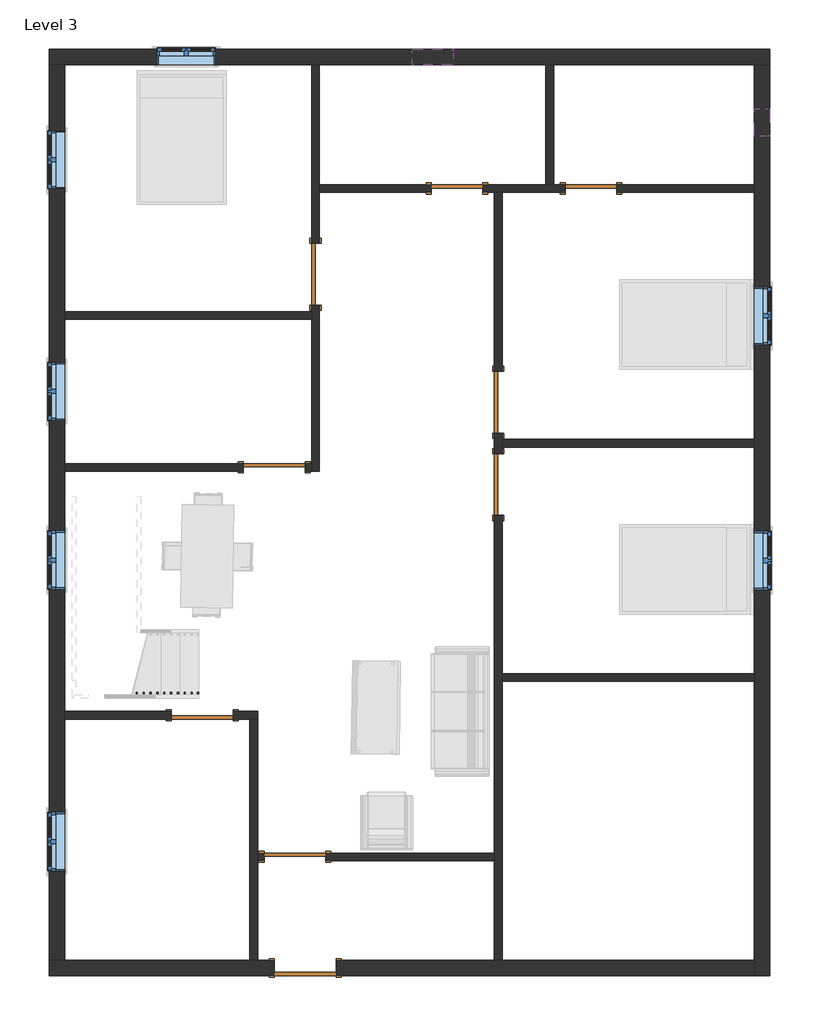
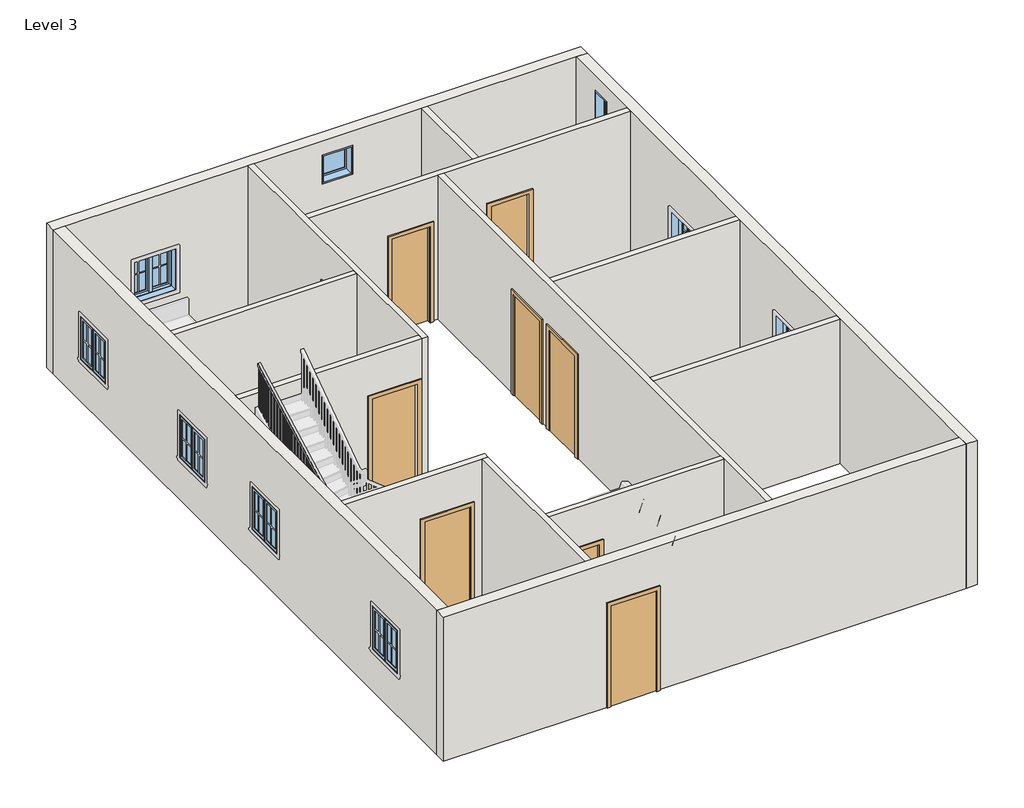
# One storey, part 1 of 2: 15 walls, 9 doors, 9 windows, 1 railing.
"""IFC4 building model written with IfcOpenShell, lengths in millimetres."""

from ifc_helpers import new_model, si_unit, frame, origin, place, context, project, spatial, polyline, outline, extrude, faceted_brep, transform, mapped, element, save
from components import door_d8f5dbb5, door_f2b275c1, door_305aa2a5, door_e5f9f3c4, door_0ca8825f, window_aa618e30, window_80340324, window_339605e1

model = new_model("IFC4")

# Units and contexts
model_context = context("Model", 3, world=origin())
ifc_project = project(units=[si_unit("LENGTHUNIT", "METRE", prefix="MILLI")], contexts=[model_context])

# Site, building, storey
site = spatial("IfcSite", under=ifc_project)
building = spatial("IfcBuilding", under=site)
storey = spatial("IfcBuildingStorey", under=building, Name="Level 3", Elevation=3200.4)

# Doors
placement = place(None, origin())
door_shape = door_d8f5dbb5(model_context)
element("IfcDoor", 1, ObjectType="Single-Flush : 30\" x 80\"", at=placement, inside=storey, context=model_context, shape_type="MappedRepresentation", body=[
    mapped(door_shape, transform((-551.6099931, 5332.4435985, 3200.4), x_axis=(1.0, 0.0, 0.0), y_axis=(0.0, 1.0, 0.0), z_axis=(0.0, 0.0, 1.0))),
])
door_2_shape = door_f2b275c1(model_context)
element("IfcDoor", 2, ObjectType="Single-Flush : 30\" x 80\"", at=placement, inside=storey, context=model_context, shape_type="MappedRepresentation", body=[
    mapped(door_2_shape, transform((1429.5900069, 5332.4435985, 3200.4), x_axis=(-1.0, 0.0, 0.0), y_axis=(0.0, -1.0, 0.0), z_axis=(0.0, 0.0, 1.0))),
])
door_3_shape = door_305aa2a5(model_context)
element("IfcDoor", 3, ObjectType="Single-Flush : 36\" x 84\"", at=placement, inside=storey, context=model_context, shape_type="MappedRepresentation", body=[
    mapped(door_3_shape, transform((-2647.1099931, 4062.4435985, 3200.4), x_axis=(0.0, -1.0, 0.0), y_axis=(1.0, 0.0, 0.0), z_axis=(0.0, 0.0, 1.0))),
])
element("IfcDoor", 4, ObjectType="Single-Flush : 36\" x 84\"", at=placement, inside=storey, context=model_context, shape_type="MappedRepresentation", body=[
    mapped(door_3_shape, transform((57.9900069, 2170.1435985, 3200.4), x_axis=(0.0, -1.0, 0.0), y_axis=(1.0, 0.0, 0.0), z_axis=(0.0, 0.0, 1.0))),
])
element("IfcDoor", 5, ObjectType="Single-Flush : 36\" x 84\"", at=placement, inside=storey, context=model_context, shape_type="MappedRepresentation", body=[
    mapped(door_3_shape, transform((-4323.5099931, -2465.3564015, 3200.4), x_axis=(1.0, 0.0, 0.0), y_axis=(0.0, 1.0, 0.0), z_axis=(0.0, 0.0, 1.0))),
])
element("IfcDoor", 6, ObjectType="Single-Flush : 36\" x 84\"", at=placement, inside=storey, context=model_context, shape_type="MappedRepresentation", body=[
    mapped(door_3_shape, transform((-2951.9099931, -4560.8564015, 3200.4), x_axis=(-1.0, 0.0, 0.0), y_axis=(0.0, -1.0, 0.0), z_axis=(0.0, 0.0, 1.0))),
])
door_4_shape = door_e5f9f3c4(model_context)
element("IfcDoor", 7, ObjectType="Single-Flush : 36\" x 84\"", at=placement, inside=storey, context=model_context, shape_type="MappedRepresentation", body=[
    mapped(door_4_shape, transform((-3256.7099931, 1204.9435985, 3200.4), x_axis=(1.0, 0.0, 0.0), y_axis=(0.0, 1.0, 0.0), z_axis=(0.0, 0.0, 1.0))),
])
element("IfcDoor", 8, ObjectType="Single-Flush : 36\" x 84\"", at=placement, inside=storey, context=model_context, shape_type="MappedRepresentation", body=[
    mapped(door_4_shape, transform((57.9900069, 950.9435985, 3200.4), x_axis=(0.0, 1.0, 0.0), y_axis=(-1.0, 0.0, 0.0), z_axis=(0.0, 0.0, 1.0))),
])
door_5_shape = door_0ca8825f(model_context)
element("IfcDoor", 9, ObjectType="Single-Flush : 36\" x 84\"", at=placement, inside=storey, context=model_context, shape_type="MappedRepresentation", body=[
    mapped(door_5_shape, transform((-2799.5099931, -6205.5064015, 3200.4), x_axis=(-1.0, 0.0, 0.0), y_axis=(0.0, -1.0, 0.0), z_axis=(0.0, 0.0, 1.0))),
])

# Railing
element("IfcRailing", 10, ObjectType="Handrail - Rectangular", at=placement, inside=storey, context=model_context, shape_type="SolidModel", body=[
    faceted_brep([(-4378.4230036, -2160.5564015, 4961.4666667), (-4378.4230036, -2160.5564015, 4905.3107192), (-4378.4230036, -2109.7564015, 4905.3107192), (-4378.4230036, -2109.7564015, 4961.4666667), (-5973.5005957, -2160.5564015, 5712.9835228), (-5984.8684735, -2160.5564015, 5662.1835228), (-5984.8684735, -2109.7564015, 5662.1835228), (-5973.5005957, -2109.7564015, 5712.9835228), (-6196.7599931, -2160.5564015, 5712.9835228), (-6196.7599931, -2160.5564015, 5662.1835228), (-6145.9599931, -2109.7564015, 5662.1835228), (-6145.9599931, -2109.7564015, 5712.9835228), (-6196.7599931, -1959.3194067, 5712.9835228), (-6196.7599931, -1946.6862419, 5662.1835228), (-6145.9599931, -1946.6862419, 5662.1835228), (-6145.9599931, -1959.3194067, 5712.9835228), (-6196.7599931, 775.380588, 7162.8), (-6145.9599931, 775.380588, 7162.8), (-6145.9599931, 775.380588, 7105.3024571), (-6196.7599931, 775.380588, 7105.3024571)], [[[0, 1, 2, 3]], [[1, 0, 4, 5]], [[2, 1, 5, 6]], [[3, 2, 6, 7]], [[0, 3, 7, 4]], [[5, 4, 8, 9]], [[6, 5, 9, 10]], [[7, 6, 10, 11]], [[4, 7, 11, 8]], [[9, 8, 12, 13]], [[10, 9, 13, 14]], [[11, 10, 14, 15]], [[8, 11, 15, 12]], [[16, 17, 18, 19]], [[13, 12, 16, 19]], [[14, 13, 19, 18]], [[15, 14, 18, 17]], [[12, 15, 17, 16]]]),
    extrude(outline(polyline([(719.1685985, 7075.5013569), (719.1685985, 6079.0666667), (700.1185985, 6079.0666667), (700.1185985, 7065.401893), (719.1685985, 7075.5013569)])), frame((-6180.8849931, 0.0, 0.0), z_axis=(1.0, 0.0, 0.0), x_axis=(0.0, 1.0, 0.0)), (0.0, 0.0, 1.0), 19.05),
    extrude(outline(polyline([(617.5685985, 7021.6375494), (617.5685985, 6079.0666667), (598.5185985, 6079.0666667), (598.5185985, 7011.5380855), (617.5685985, 7021.6375494)])), frame((-6180.8849931, 0.0, 0.0), z_axis=(1.0, 0.0, 0.0), x_axis=(0.0, 1.0, 0.0)), (0.0, 0.0, 1.0), 19.05),
    extrude(outline(polyline([(515.9685985, 6967.7737419), (515.9685985, 6079.0666667), (496.9185985, 6079.0666667), (496.9185985, 6957.674278), (515.9685985, 6967.7737419)])), frame((-6180.8849931, 0.0, 0.0), z_axis=(1.0, 0.0, 0.0), x_axis=(0.0, 1.0, 0.0)), (0.0, 0.0, 1.0), 19.05),
    extrude(outline(polyline([(414.3685985, 6913.9099344), (414.3685985, 5909.7333333), (395.3185985, 5909.7333333), (395.3185985, 6903.8104705), (414.3685985, 6913.9099344)])), frame((-6180.8849931, 0.0, 0.0), z_axis=(1.0, 0.0, 0.0), x_axis=(0.0, 1.0, 0.0)), (0.0, 0.0, 1.0), 19.05),
    extrude(outline(polyline([(312.7685985, 6860.0461269), (312.7685985, 5909.7333333), (293.7185985, 5909.7333333), (293.7185985, 6849.946663), (312.7685985, 6860.0461269)])), frame((-6180.8849931, 0.0, 0.0), z_axis=(1.0, 0.0, 0.0), x_axis=(0.0, 1.0, 0.0)), (0.0, 0.0, 1.0), 19.05),
    extrude(outline(polyline([(211.1685985, 6806.1823194), (211.1685985, 5740.4), (192.1185985, 5740.4), (192.1185985, 6796.0828555), (211.1685985, 6806.1823194)])), frame((-6180.8849931, 0.0, 0.0), z_axis=(1.0, 0.0, 0.0), x_axis=(0.0, 1.0, 0.0)), (0.0, 0.0, 1.0), 19.05),
    extrude(outline(polyline([(109.5685985, 6752.3185119), (109.5685985, 5740.4), (90.5185985, 5740.4), (90.5185985, 6742.219048), (109.5685985, 6752.3185119)])), frame((-6180.8849931, 0.0, 0.0), z_axis=(1.0, 0.0, 0.0), x_axis=(0.0, 1.0, 0.0)), (0.0, 0.0, 1.0), 19.05),
    extrude(outline(polyline([(7.9685985, 6698.4547044), (7.9685985, 5740.4), (-11.0814015, 5740.4), (-11.0814015, 6688.3552405), (7.9685985, 6698.4547044)])), frame((-6180.8849931, 0.0, 0.0), z_axis=(1.0, 0.0, 0.0), x_axis=(0.0, 1.0, 0.0)), (0.0, 0.0, 1.0), 19.05),
    extrude(outline(polyline([(-93.6314015, 6644.5908969), (-93.6314015, 5571.0666667), (-112.6814015, 5571.0666667), (-112.6814015, 6634.491433), (-93.6314015, 6644.5908969)])), frame((-6180.8849931, 0.0, 0.0), z_axis=(1.0, 0.0, 0.0), x_axis=(0.0, 1.0, 0.0)), (0.0, 0.0, 1.0), 19.05),
    extrude(outline(polyline([(-195.2314015, 6590.7270894), (-195.2314015, 5571.0666667), (-214.2814015, 5571.0666667), (-214.2814015, 6580.6276255), (-195.2314015, 6590.7270894)])), frame((-6180.8849931, 0.0, 0.0), z_axis=(1.0, 0.0, 0.0), x_axis=(0.0, 1.0, 0.0)), (0.0, 0.0, 1.0), 19.05),
    extrude(outline(polyline([(-296.8314015, 6536.8632819), (-296.8314015, 5571.0666667), (-315.8814015, 5571.0666667), (-315.8814015, 6526.763818), (-296.8314015, 6536.8632819)])), frame((-6180.8849931, 0.0, 0.0), z_axis=(1.0, 0.0, 0.0), x_axis=(0.0, 1.0, 0.0)), (0.0, 0.0, 1.0), 19.05),
    extrude(outline(polyline([(-398.4314015, 6482.9994744), (-398.4314015, 5401.7333333), (-417.4814015, 5401.7333333), (-417.4814015, 6472.9000105), (-398.4314015, 6482.9994744)])), frame((-6180.8849931, 0.0, 0.0), z_axis=(1.0, 0.0, 0.0), x_axis=(0.0, 1.0, 0.0)), (0.0, 0.0, 1.0), 19.05),
    extrude(outline(polyline([(-500.0314015, 6429.1356669), (-500.0314015, 5401.7333333), (-519.0814015, 5401.7333333), (-519.0814015, 6419.036203), (-500.0314015, 6429.1356669)])), frame((-6180.8849931, 0.0, 0.0), z_axis=(1.0, 0.0, 0.0), x_axis=(0.0, 1.0, 0.0)), (0.0, 0.0, 1.0), 19.05),
    extrude(outline(polyline([(-601.6314015, 6375.2718594), (-601.6314015, 5401.7333333), (-620.6814015, 5401.7333333), (-620.6814015, 6365.1723955), (-601.6314015, 6375.2718594)])), frame((-6180.8849931, 0.0, 0.0), z_axis=(1.0, 0.0, 0.0), x_axis=(0.0, 1.0, 0.0)), (0.0, 0.0, 1.0), 19.05),
    extrude(outline(polyline([(-703.2314015, 6321.4080519), (-703.2314015, 5232.4), (-722.2814015, 5232.4), (-722.2814015, 6311.308588), (-703.2314015, 6321.4080519)])), frame((-6180.8849931, 0.0, 0.0), z_axis=(1.0, 0.0, 0.0), x_axis=(0.0, 1.0, 0.0)), (0.0, 0.0, 1.0), 19.05),
    extrude(outline(polyline([(-804.8314015, 6267.5442444), (-804.8314015, 5232.4), (-823.8814015, 5232.4), (-823.8814015, 6257.4447805), (-804.8314015, 6267.5442444)])), frame((-6180.8849931, 0.0, 0.0), z_axis=(1.0, 0.0, 0.0), x_axis=(0.0, 1.0, 0.0)), (0.0, 0.0, 1.0), 19.05),
    extrude(outline(polyline([(-906.4314015, 6213.6804369), (-906.4314015, 5232.4), (-925.4814015, 5232.4), (-925.4814015, 6203.580973), (-906.4314015, 6213.6804369)])), frame((-6180.8849931, 0.0, 0.0), z_axis=(1.0, 0.0, 0.0), x_axis=(0.0, 1.0, 0.0)), (0.0, 0.0, 1.0), 19.05),
    extrude(outline(polyline([(-1008.0314015, 6159.8166294), (-1008.0314015, 5063.0666667), (-1027.0814015, 5063.0666667), (-1027.0814015, 6149.7171655), (-1008.0314015, 6159.8166294)])), frame((-6180.8849931, 0.0, 0.0), z_axis=(1.0, 0.0, 0.0), x_axis=(0.0, 1.0, 0.0)), (0.0, 0.0, 1.0), 19.05),
    extrude(outline(polyline([(-1109.6314015, 6105.9528219), (-1109.6314015, 5063.0666667), (-1128.6814015, 5063.0666667), (-1128.6814015, 6095.853358), (-1109.6314015, 6105.9528219)])), frame((-6180.8849931, 0.0, 0.0), z_axis=(1.0, 0.0, 0.0), x_axis=(0.0, 1.0, 0.0)), (0.0, 0.0, 1.0), 19.05),
    extrude(outline(polyline([(-1211.2314015, 6052.0890144), (-1211.2314015, 5063.0666667), (-1230.2814015, 5063.0666667), (-1230.2814015, 6041.9895505), (-1211.2314015, 6052.0890144)])), frame((-6180.8849931, 0.0, 0.0), z_axis=(1.0, 0.0, 0.0), x_axis=(0.0, 1.0, 0.0)), (0.0, 0.0, 1.0), 19.05),
    extrude(outline(polyline([(-1312.8314015, 5998.2252069), (-1312.8314015, 5063.0666667), (-1331.8814015, 5063.0666667), (-1331.8814015, 5988.125743), (-1312.8314015, 5998.2252069)])), frame((-6180.8849931, 0.0, 0.0), z_axis=(1.0, 0.0, 0.0), x_axis=(0.0, 1.0, 0.0)), (0.0, 0.0, 1.0), 19.05),
    extrude(outline(polyline([(-1414.4314015, 5944.3613994), (-1414.4314015, 4893.7333333), (-1433.4814015, 4893.7333333), (-1433.4814015, 5934.2619355), (-1414.4314015, 5944.3613994)])), frame((-6180.8849931, 0.0, 0.0), z_axis=(1.0, 0.0, 0.0), x_axis=(0.0, 1.0, 0.0)), (0.0, 0.0, 1.0), 19.05),
    extrude(outline(polyline([(-1516.0314015, 5890.4975919), (-1516.0314015, 4893.7333333), (-1535.0814015, 4893.7333333), (-1535.0814015, 5880.398128), (-1516.0314015, 5890.4975919)])), frame((-6180.8849931, 0.0, 0.0), z_axis=(1.0, 0.0, 0.0), x_axis=(0.0, 1.0, 0.0)), (0.0, 0.0, 1.0), 19.05),
    extrude(outline(polyline([(-1617.6314015, 5836.6337844), (-1617.6314015, 4893.7333333), (-1636.6814015, 4893.7333333), (-1636.6814015, 5826.5343205), (-1617.6314015, 5836.6337844)])), frame((-6180.8849931, 0.0, 0.0), z_axis=(1.0, 0.0, 0.0), x_axis=(0.0, 1.0, 0.0)), (0.0, 0.0, 1.0), 19.05),
    extrude(outline(polyline([(-1719.2314015, 5782.7699769), (-1719.2314015, 4893.7333333), (-1738.2814015, 4893.7333333), (-1738.2814015, 5772.670513), (-1719.2314015, 5782.7699769)])), frame((-6180.8849931, 0.0, 0.0), z_axis=(1.0, 0.0, 0.0), x_axis=(0.0, 1.0, 0.0)), (0.0, 0.0, 1.0), 19.05),
    extrude(outline(polyline([(-1820.8314015, 5728.9061694), (-1820.8314015, 4724.4), (-1839.8814015, 4724.4), (-1839.8814015, 5718.8067055), (-1820.8314015, 5728.9061694)])), frame((-6180.8849931, 0.0, 0.0), z_axis=(1.0, 0.0, 0.0), x_axis=(0.0, 1.0, 0.0)), (0.0, 0.0, 1.0), 19.05),
    extrude(outline(polyline([(-1922.4314015, 5675.0423619), (-1922.4314015, 4724.4), (-1941.4814015, 4724.4), (-1941.4814015, 5664.942898), (-1922.4314015, 5675.0423619)])), frame((-6180.8849931, 0.0, 0.0), z_axis=(1.0, 0.0, 0.0), x_axis=(0.0, 1.0, 0.0)), (0.0, 0.0, 1.0), 19.05),
    extrude(outline(polyline([(-6180.8849931, -2043.0814015), (-6180.8849931, -2024.0314015), (-6161.8349931, -2024.0314015), (-6161.8349931, -2043.0814015), (-6180.8849931, -2043.0814015)])), frame((0.0, 0.0, 4724.4), z_axis=(0.0, 0.0, 1.0), x_axis=(1.0, 0.0, 0.0)), (0.0, 0.0, 1.0), 937.7835228),
    extrude(outline(polyline([(-6096.0980036, -2144.6814015), (-6115.1480036, -2144.6814015), (-6115.1480036, -2125.6314015), (-6096.0980036, -2125.6314015), (-6096.0980036, -2144.6814015)])), frame((0.0, 0.0, 4724.4), z_axis=(0.0, 0.0, 1.0), x_axis=(1.0, 0.0, 0.0)), (0.0, 0.0, 1.0), 937.7835228),
    extrude(outline(polyline([(-5994.4980036, -2144.6814015), (-6013.5480036, -2144.6814015), (-6013.5480036, -2125.6314015), (-5994.4980036, -2125.6314015), (-5994.4980036, -2144.6814015)])), frame((0.0, 0.0, 4724.4), z_axis=(0.0, 0.0, 1.0), x_axis=(1.0, 0.0, 0.0)), (0.0, 0.0, 1.0), 937.7835228),
    extrude(outline(polyline([(5627.827224, -5911.9480036), (4724.4, -5911.9480036), (4724.4, -5892.8980036), (5618.8518637, -5892.8980036), (5627.827224, -5911.9480036)])), frame((0.0, -2144.6814015, 0.0), z_axis=(0.0, 1.0, 0.0), x_axis=(0.0, 0.0, 1.0)), (0.0, 0.0, 1.0), 19.05),
    extrude(outline(polyline([(5579.9586357, -5810.3480036), (4724.4, -5810.3480036), (4724.4, -5791.2980036), (5570.9832754, -5791.2980036), (5579.9586357, -5810.3480036)])), frame((0.0, -2144.6814015, 0.0), z_axis=(0.0, 1.0, 0.0), x_axis=(0.0, 0.0, 1.0)), (0.0, 0.0, 1.0), 19.05),
    extrude(outline(polyline([(5532.0900474, -5708.7480036), (4555.0666667, -5708.7480036), (4555.0666667, -5689.6980036), (5523.1146871, -5689.6980036), (5532.0900474, -5708.7480036)])), frame((0.0, -2144.6814015, 0.0), z_axis=(0.0, 1.0, 0.0), x_axis=(0.0, 0.0, 1.0)), (0.0, 0.0, 1.0), 19.05),
    extrude(outline(polyline([(5484.2214591, -5607.1480036), (4555.0666667, -5607.1480036), (4555.0666667, -5588.0980036), (5475.2460988, -5588.0980036), (5484.2214591, -5607.1480036)])), frame((0.0, -2144.6814015, 0.0), z_axis=(0.0, 1.0, 0.0), x_axis=(0.0, 0.0, 1.0)), (0.0, 0.0, 1.0), 19.05),
    extrude(outline(polyline([(5436.3528708, -5505.5480036), (4555.0666667, -5505.5480036), (4555.0666667, -5486.4980036), (5427.3775105, -5486.4980036), (5436.3528708, -5505.5480036)])), frame((0.0, -2144.6814015, 0.0), z_axis=(0.0, 1.0, 0.0), x_axis=(0.0, 0.0, 1.0)), (0.0, 0.0, 1.0), 19.05),
    extrude(outline(polyline([(5388.4842825, -5403.9480036), (4555.0666667, -5403.9480036), (4555.0666667, -5384.8980036), (5379.5089222, -5384.8980036), (5388.4842825, -5403.9480036)])), frame((0.0, -2144.6814015, 0.0), z_axis=(0.0, 1.0, 0.0), x_axis=(0.0, 0.0, 1.0)), (0.0, 0.0, 1.0), 19.05),
    extrude(outline(polyline([(5340.6156942, -5302.3480036), (4385.7333333, -5302.3480036), (4385.7333333, -5283.2980036), (5331.6403338, -5283.2980036), (5340.6156942, -5302.3480036)])), frame((0.0, -2144.6814015, 0.0), z_axis=(0.0, 1.0, 0.0), x_axis=(0.0, 0.0, 1.0)), (0.0, 0.0, 1.0), 19.05),
    extrude(outline(polyline([(5292.7471058, -5200.7480036), (4385.7333333, -5200.7480036), (4385.7333333, -5181.6980036), (5283.7717455, -5181.6980036), (5292.7471058, -5200.7480036)])), frame((0.0, -2144.6814015, 0.0), z_axis=(0.0, 1.0, 0.0), x_axis=(0.0, 0.0, 1.0)), (0.0, 0.0, 1.0), 19.05),
    extrude(outline(polyline([(5244.8785175, -5099.1480036), (4385.7333333, -5099.1480036), (4385.7333333, -5080.0980036), (5235.9031572, -5080.0980036), (5244.8785175, -5099.1480036)])), frame((0.0, -2144.6814015, 0.0), z_axis=(0.0, 1.0, 0.0), x_axis=(0.0, 0.0, 1.0)), (0.0, 0.0, 1.0), 19.05),
    extrude(outline(polyline([(5197.0099292, -4997.5480036), (4385.7333333, -4997.5480036), (4385.7333333, -4978.4980036), (5188.0345689, -4978.4980036), (5197.0099292, -4997.5480036)])), frame((0.0, -2144.6814015, 0.0), z_axis=(0.0, 1.0, 0.0), x_axis=(0.0, 0.0, 1.0)), (0.0, 0.0, 1.0), 19.05),
    extrude(outline(polyline([(5149.1413409, -4895.9480036), (4216.4, -4895.9480036), (4216.4, -4876.8980036), (5140.1659806, -4876.8980036), (5149.1413409, -4895.9480036)])), frame((0.0, -2144.6814015, 0.0), z_axis=(0.0, 1.0, 0.0), x_axis=(0.0, 0.0, 1.0)), (0.0, 0.0, 1.0), 19.05),
    extrude(outline(polyline([(5101.2727526, -4794.3480036), (4216.4, -4794.3480036), (4216.4, -4775.2980036), (5092.2973923, -4775.2980036), (5101.2727526, -4794.3480036)])), frame((0.0, -2144.6814015, 0.0), z_axis=(0.0, 1.0, 0.0), x_axis=(0.0, 0.0, 1.0)), (0.0, 0.0, 1.0), 19.05),
    extrude(outline(polyline([(5053.4041643, -4692.7480036), (4216.4, -4692.7480036), (4216.4, -4673.6980036), (5044.428804, -4673.6980036), (5053.4041643, -4692.7480036)])), frame((0.0, -2144.6814015, 0.0), z_axis=(0.0, 1.0, 0.0), x_axis=(0.0, 0.0, 1.0)), (0.0, 0.0, 1.0), 19.05),
    extrude(outline(polyline([(5005.535576, -4591.1480036), (4047.0666667, -4591.1480036), (4047.0666667, -4572.0980036), (4996.5602157, -4572.0980036), (5005.535576, -4591.1480036)])), frame((0.0, -2144.6814015, 0.0), z_axis=(0.0, 1.0, 0.0), x_axis=(0.0, 0.0, 1.0)), (0.0, 0.0, 1.0), 19.05),
    extrude(outline(polyline([(4957.6669877, -4489.5480036), (4047.0666667, -4489.5480036), (4047.0666667, -4470.4980036), (4948.6916273, -4470.4980036), (4957.6669877, -4489.5480036)])), frame((0.0, -2144.6814015, 0.0), z_axis=(0.0, 1.0, 0.0), x_axis=(0.0, 0.0, 1.0)), (0.0, 0.0, 1.0), 19.05),
    extrude(outline(polyline([(-6161.8349931, -2144.6814015), (-6180.8849931, -2144.6814015), (-6180.8849931, -2125.6314015), (-6161.8349931, -2125.6314015), (-6161.8349931, -2144.6814015)])), frame((0.0, 0.0, 4724.4), z_axis=(0.0, 0.0, 1.0), x_axis=(1.0, 0.0, 0.0)), (0.0, 0.0, 1.0), 937.7835228),
    extrude(outline(polyline([(775.380588, 7105.3024571), (775.380588, 6079.0666667), (756.330588, 6079.0666667), (756.330588, 7095.2029932), (775.380588, 7105.3024571)])), frame((-6180.8849931, 0.0, 0.0), z_axis=(1.0, 0.0, 0.0), x_axis=(0.0, 1.0, 0.0)), (0.0, 0.0, 1.0), 19.05),
    extrude(outline(polyline([(4914.2860795, -4397.4730036), (4047.0666667, -4397.4730036), (4047.0666667, -4378.4230036), (4905.3107192, -4378.4230036), (4914.2860795, -4397.4730036)])), frame((0.0, -2144.6814015, 0.0), z_axis=(0.0, 1.0, 0.0), x_axis=(0.0, 0.0, 1.0)), (0.0, 0.0, 1.0), 19.05),
])

# Walls
element("IfcWall", 11, ObjectType="WALL4.5\"", at=placement, inside=storey, context=model_context, shape_type="SweptSolid", body=[
    extrude(outline(polyline([(-2704.2599931, 3395.6935985), (-6361.8599931, 3395.6935985), (-6361.8599931, 3509.9935985), (-2704.2599931, 3509.9935985), (-2704.2599931, 3395.6935985)])), frame((0.0, 0.0, 3200.4), z_axis=(0.0, 0.0, 1.0), x_axis=(1.0, 0.0, 0.0)), (0.0, 0.0, 1.0), 3048.0),
])
element("IfcWall", 12, ObjectType="WALL4.5\"", at=placement, inside=storey, context=model_context, shape_type="Brep", body=[
    faceted_brep([(-2704.2599931, 3605.2435985, 5334.0), (-2704.2599931, 3605.2435985, 3200.4), (-2704.2599931, 3509.9935985, 3200.4), (-2704.2599931, 3395.6935985, 3200.4), (-2704.2599931, 1262.0935985, 3200.4), (-2704.2599931, 1147.7935985, 3200.4), (-2704.2599931, 1147.7935985, 6248.4), (-2704.2599931, 1262.0935985, 6248.4), (-2704.2599931, 3395.6935985, 6248.4), (-2704.2599931, 3509.9935985, 6248.4), (-2704.2599931, 7167.5935985, 6248.4), (-2704.2599931, 7167.5935985, 3200.4), (-2704.2599931, 4519.6435985, 3200.4), (-2704.2599931, 4519.6435985, 5334.0), (-2589.9599931, 1147.7935985, 3200.4), (-2589.9599931, 3605.2435985, 3200.4), (-2589.9599931, 3605.2435985, 5334.0), (-2589.9599931, 4519.6435985, 5334.0), (-2589.9599931, 4519.6435985, 3200.4), (-2589.9599931, 5275.2935985, 3200.4), (-2589.9599931, 5389.5935985, 3200.4), (-2589.9599931, 7167.5935985, 3200.4), (-2589.9599931, 7167.5935985, 6248.4), (-2589.9599931, 5389.5935985, 6248.4), (-2589.9599931, 5275.2935985, 6248.4), (-2589.9599931, 1147.7935985, 6248.4)], [[[0, 1, 2, 3, 4, 5, 6, 7, 8, 9, 10, 11, 12, 13]], [[14, 15, 16, 17, 18, 19, 20, 21, 22, 23, 24, 25]], [[12, 11, 21, 20, 19, 18]], [[5, 4, 3, 2, 1, 15, 14]], [[11, 10, 22, 21]], [[6, 5, 14, 25]], [[16, 15, 1, 0]], [[17, 16, 0, 13]], [[18, 17, 13, 12]], [[10, 9, 8, 7, 6, 25, 24, 23, 22]]]),
])
element("IfcWall", 13, ObjectType="WALL4.5\"", at=placement, inside=storey, context=model_context, shape_type="SweptSolid", body=[
    extrude(outline(polyline([(5334.0, -2799.5099931), (3200.4, -2799.5099931), (3200.4, -2704.2599931), (6248.4, -2704.2599931), (6248.4, -6361.8599931), (3200.4, -6361.8599931), (3200.4, -3713.9099931), (5334.0, -3713.9099931), (5334.0, -2799.5099931)])), frame((0.0, 1147.7935985, 0.0), z_axis=(0.0, 1.0, 0.0), x_axis=(0.0, 0.0, 1.0)), (0.0, 0.0, 1.0), 114.3),
])
element("IfcWall", 14, ObjectType="WALL4.5\"", at=placement, inside=storey, context=model_context, shape_type="Brep", body=[
    faceted_brep([(-170.6099931, 5275.2935985, 3200.4), (0.8400069, 5275.2935985, 3200.4), (115.1400069, 5275.2935985, 3200.4), (1048.5900069, 5275.2935985, 3200.4), (1048.5900069, 5275.2935985, 5232.4), (1810.5900069, 5275.2935985, 5232.4), (1810.5900069, 5275.2935985, 3200.4), (3848.9400069, 5275.2935985, 3200.4), (3848.9400069, 5275.2935985, 6248.4), (115.1400069, 5275.2935985, 6248.4), (0.8400069, 5275.2935985, 6248.4), (-2589.9599931, 5275.2935985, 6248.4), (-2589.9599931, 5275.2935985, 3200.4), (-932.6099931, 5275.2935985, 3200.4), (-932.6099931, 5275.2935985, 5232.4), (-170.6099931, 5275.2935985, 5232.4), (1048.5900069, 5389.5935985, 5232.4), (1048.5900069, 5389.5935985, 3200.4), (877.1400069, 5389.5935985, 3200.4), (762.8400069, 5389.5935985, 3200.4), (-170.6099931, 5389.5935985, 3200.4), (-170.6099931, 5389.5935985, 5232.4), (-932.6099931, 5389.5935985, 5232.4), (-932.6099931, 5389.5935985, 3200.4), (-2589.9599931, 5389.5935985, 3200.4), (-2589.9599931, 5389.5935985, 6248.4), (762.8400069, 5389.5935985, 6248.4), (877.1400069, 5389.5935985, 6248.4), (3848.9400069, 5389.5935985, 6248.4), (3848.9400069, 5389.5935985, 3200.4), (1810.5900069, 5389.5935985, 3200.4), (1810.5900069, 5389.5935985, 5232.4)], [[[0, 1, 2, 3, 4, 5, 6, 7, 8, 9, 10, 11, 12, 13, 14, 15]], [[16, 17, 18, 19, 20, 21, 22, 23, 24, 25, 26, 27, 28, 29, 30, 31]], [[13, 12, 24, 23]], [[30, 29, 7, 6]], [[20, 19, 18, 17, 3, 2, 1, 0]], [[8, 7, 29, 28]], [[12, 11, 25, 24]], [[21, 20, 0, 15]], [[22, 21, 15, 14]], [[23, 22, 14, 13]], [[4, 3, 17, 16]], [[5, 4, 16, 31]], [[6, 5, 31, 30]], [[11, 10, 9, 8, 28, 27, 26, 25]]]),
])
element("IfcWall", 15, ObjectType="WALL4.5\"", at=placement, inside=storey, context=model_context, shape_type="SweptSolid", body=[
    extrude(outline(polyline([(762.8400069, 5389.5935985), (762.8400069, 7167.5935985), (877.1400069, 7167.5935985), (877.1400069, 5389.5935985), (762.8400069, 5389.5935985)])), frame((0.0, 0.0, 3200.4), z_axis=(0.0, 0.0, 1.0), x_axis=(1.0, 0.0, 0.0)), (0.0, 0.0, 1.0), 3048.0),
])
element("IfcWall", 16, ObjectType="WALL4.5\"", at=placement, inside=storey, context=model_context, shape_type="Brep", body=[
    faceted_brep([(0.8400069, 1712.9435985, 3200.4), (0.8400069, 1408.1435985, 3200.4), (0.8400069, 1408.1435985, 5334.0), (0.8400069, 493.7435985, 5334.0), (0.8400069, 493.7435985, 3200.4), (0.8400069, -4503.7064015, 3200.4), (0.8400069, -4618.0064015, 3200.4), (0.8400069, -6091.2064015, 3200.4), (0.8400069, -6091.2064015, 6248.4), (0.8400069, -4618.0064015, 6248.4), (0.8400069, -4503.7064015, 6248.4), (0.8400069, 5275.2935985, 6248.4), (0.8400069, 5275.2935985, 3200.4), (0.8400069, 2627.3435985, 3200.4), (0.8400069, 2627.3435985, 5334.0), (0.8400069, 1712.9435985, 5334.0), (115.1400069, 1408.1435985, 5334.0), (115.1400069, 1408.1435985, 3200.4), (115.1400069, 1503.3935985, 3200.4), (115.1400069, 1617.6935985, 3200.4), (115.1400069, 1712.9435985, 3200.4), (115.1400069, 1712.9435985, 5334.0), (115.1400069, 2627.3435985, 5334.0), (115.1400069, 2627.3435985, 3200.4), (115.1400069, 5275.2935985, 3200.4), (115.1400069, 5275.2935985, 6248.4), (115.1400069, 1617.6935985, 6248.4), (115.1400069, 1503.3935985, 6248.4), (115.1400069, -1850.058017, 6248.4), (115.1400069, -1964.358017, 6248.4), (115.1400069, -6091.2064015, 6248.4), (115.1400069, -6091.2064015, 3200.4), (115.1400069, -1964.358017, 3200.4), (115.1400069, -1850.058017, 3200.4), (115.1400069, 493.7435985, 3200.4), (115.1400069, 493.7435985, 5334.0)], [[[0, 1, 2, 3, 4, 5, 6, 7, 8, 9, 10, 11, 12, 13, 14, 15]], [[16, 17, 18, 19, 20, 21, 22, 23, 24, 25, 26, 27, 28, 29, 30, 31, 32, 33, 34, 35]], [[13, 12, 24, 23]], [[34, 33, 32, 31, 7, 6, 5, 4]], [[20, 19, 18, 17, 1, 0]], [[8, 7, 31, 30]], [[12, 11, 25, 24]], [[21, 20, 0, 15]], [[22, 21, 15, 14]], [[23, 22, 14, 13]], [[2, 1, 17, 16]], [[3, 2, 16, 35]], [[4, 3, 35, 34]], [[11, 10, 9, 8, 30, 29, 28, 27, 26, 25]]]),
])
element("IfcWall", 17, ObjectType="WALL4.5\"", at=placement, inside=storey, context=model_context, shape_type="SweptSolid", body=[
    extrude(outline(polyline([(3848.9400069, -1964.358017), (115.1400069, -1964.358017), (115.1400069, -1850.058017), (3848.9400069, -1850.058017), (3848.9400069, -1964.358017)])), frame((0.0, 0.0, 3200.4), z_axis=(0.0, 0.0, 1.0), x_axis=(1.0, 0.0, 0.0)), (0.0, 0.0, 1.0), 3048.0),
])
element("IfcWall", 18, ObjectType="WALL4.5\"", at=placement, inside=storey, context=model_context, shape_type="SweptSolid", body=[
    extrude(outline(polyline([(3848.9400069, 1503.3935985), (115.1400069, 1503.3935985), (115.1400069, 1617.6935985), (3848.9400069, 1617.6935985), (3848.9400069, 1503.3935985)])), frame((0.0, 0.0, 3200.4), z_axis=(0.0, 0.0, 1.0), x_axis=(1.0, 0.0, 0.0)), (0.0, 0.0, 1.0), 3048.0),
])
element("IfcWall", 19, ObjectType="WALL4.5\"", at=placement, inside=storey, context=model_context, shape_type="Brep", body=[
    faceted_brep([(-3866.3099931, -2522.5064015, 5334.0), (-3866.3099931, -2522.5064015, 3200.4), (-3618.6599931, -2522.5064015, 3200.4), (-3504.3599931, -2522.5064015, 3200.4), (-3504.3599931, -2522.5064015, 6248.4), (-3618.6599931, -2522.5064015, 6248.4), (-6361.8599931, -2522.5064015, 6248.4), (-6361.8599931, -2522.5064015, 3200.4), (-4780.7099931, -2522.5064015, 3200.4), (-4780.7099931, -2522.5064015, 5334.0), (-3504.3599931, -2408.2064015, 3200.4), (-3866.3099931, -2408.2064015, 3200.4), (-3866.3099931, -2408.2064015, 5334.0), (-4780.7099931, -2408.2064015, 5334.0), (-4780.7099931, -2408.2064015, 3200.4), (-6361.8599931, -2408.2064015, 3200.4), (-6361.8599931, -2408.2064015, 6248.4), (-3504.3599931, -2408.2064015, 6248.4)], [[[0, 1, 2, 3, 4, 5, 6, 7, 8, 9]], [[10, 11, 12, 13, 14, 15, 16, 17]], [[8, 7, 15, 14]], [[3, 2, 1, 11, 10]], [[7, 6, 16, 15]], [[4, 3, 10, 17]], [[12, 11, 1, 0]], [[13, 12, 0, 9]], [[14, 13, 9, 8]], [[6, 5, 4, 17, 16]]]),
])
element("IfcWall", 20, ObjectType="WALL4.5\"", at=placement, inside=storey, context=model_context, shape_type="SweptSolid", body=[
    extrude(outline(polyline([(3200.4, -3504.3599931), (3200.4, -3409.1099931), (5334.0, -3409.1099931), (5334.0, -2494.7099931), (3200.4, -2494.7099931), (3200.4, 0.8400069), (6248.4, 0.8400069), (6248.4, -3504.3599931), (3200.4, -3504.3599931)])), frame((0.0, -4618.0064015, 0.0), z_axis=(0.0, 1.0, 0.0), x_axis=(0.0, 0.0, 1.0)), (0.0, 0.0, 1.0), 114.3),
])
element("IfcWall", 21, ObjectType="WALL4.5\"", at=placement, inside=storey, context=model_context, shape_type="Brep", body=[
    faceted_brep([(-3504.3599931, -6091.2064015, 3200.4), (-3504.3599931, -4618.0064015, 3200.4), (-3504.3599931, -4503.7064015, 3200.4), (-3504.3599931, -2522.5064015, 3200.4), (-3504.3599931, -2522.5064015, 6248.4), (-3504.3599931, -4503.7064015, 6248.4), (-3504.3599931, -4618.0064015, 6248.4), (-3504.3599931, -6091.2064015, 6248.4), (-3618.6599931, -6091.2064015, 3200.4), (-3618.6599931, -6091.2064015, 6248.4), (-3618.6599931, -2522.5064015, 6248.4), (-3618.6599931, -2522.5064015, 3200.4)], [[[0, 1, 2, 3, 4, 5, 6, 7]], [[8, 9, 10, 11]], [[3, 2, 1, 0, 8, 11]], [[4, 3, 11, 10]], [[0, 7, 9, 8]], [[7, 6, 5, 4, 10, 9]]]),
])
element("IfcWall", 22, ObjectType="WALL9\"", at=placement, inside=storey, context=model_context, shape_type="Brep", body=[
    faceted_brep([(-6590.4599931, 7167.5935985, 3200.4), (-6361.8599931, 7167.5935985, 3200.4), (-2704.2599931, 7167.5935985, 3200.4), (-2589.9599931, 7167.5935985, 3200.4), (762.8400069, 7167.5935985, 3200.4), (877.1400069, 7167.5935985, 3200.4), (3848.9400069, 7167.5935985, 3200.4), (4077.5400069, 7167.5935985, 3200.4), (4077.5400069, 7167.5935985, 6248.4), (3848.9400069, 7167.5935985, 6248.4), (877.1400069, 7167.5935985, 6248.4), (762.8400069, 7167.5935985, 6248.4), (-2589.9599931, 7167.5935985, 6248.4), (-2704.2599931, 7167.5935985, 6248.4), (-6361.8599931, 7167.5935985, 6248.4), (-6590.4599931, 7167.5935985, 6248.4), (-608.7599931, 7167.5935985, 5943.6), (-608.7599931, 7167.5935985, 5334.0), (-1218.3599931, 7167.5935985, 5334.0), (-1218.3599931, 7167.5935985, 5943.6), (-4129.8349931, 7167.5935985, 5029.2), (-4129.8349931, 7167.5935985, 4114.8), (-4993.4349931, 7167.5935985, 4114.8), (-4993.4349931, 7167.5935985, 5029.2), (4077.5400069, 7396.1935985, 3200.4), (-6590.4599931, 7396.1935985, 3200.4), (-6590.4599931, 7396.1935985, 6248.4), (4077.5400069, 7396.1935985, 6248.4), (-608.7599931, 7396.1935985, 5334.0), (-608.7599931, 7396.1935985, 5943.6), (-1218.3599931, 7396.1935985, 5943.6), (-1218.3599931, 7396.1935985, 5334.0), (-4129.8349931, 7396.1935985, 4114.8), (-4129.8349931, 7396.1935985, 5029.2), (-4993.4349931, 7396.1935985, 5029.2), (-4993.4349931, 7396.1935985, 4114.8)], [[[0, 1, 2, 3, 4, 5, 6, 7, 8, 9, 10, 11, 12, 13, 14, 15], [16, 17, 18, 19], [20, 21, 22, 23]], [[24, 25, 26, 27], [28, 29, 30, 31], [32, 33, 34, 35]], [[7, 6, 5, 4, 3, 2, 1, 0, 25, 24]], [[8, 7, 24, 27]], [[0, 15, 26, 25]], [[16, 29, 28, 17]], [[17, 28, 31, 18]], [[18, 31, 30, 19]], [[21, 20, 33, 32]], [[22, 21, 32, 35]], [[23, 22, 35, 34]], [[20, 23, 34, 33]], [[15, 14, 13, 12, 11, 10, 9, 8, 27, 26]], [[29, 16, 19, 30]]]),
])
element("IfcWall", 23, ObjectType="WALL9\"", at=placement, inside=storey, context=model_context, shape_type="Brep", body=[
    faceted_brep([(3848.9400069, 7167.5935985, 3200.4), (3848.9400069, 5389.5935985, 3200.4), (3848.9400069, 5275.2935985, 3200.4), (3848.9400069, 1617.6935985, 3200.4), (3848.9400069, 1503.3935985, 3200.4), (3848.9400069, -1850.058017, 3200.4), (3848.9400069, -1964.358017, 3200.4), (3848.9400069, -6091.2064015, 3200.4), (3848.9400069, -6319.8064015, 3200.4), (3848.9400069, -6319.8064015, 6248.4), (3848.9400069, -6091.2064015, 6248.4), (3848.9400069, -1964.358017, 6248.4), (3848.9400069, -1850.058017, 6248.4), (3848.9400069, 1503.3935985, 6248.4), (3848.9400069, 1617.6935985, 6248.4), (3848.9400069, 5275.2935985, 6248.4), (3848.9400069, 5389.5935985, 6248.4), (3848.9400069, 7167.5935985, 6248.4), (3848.9400069, 6103.9685985, 5943.6), (3848.9400069, 6103.9685985, 5334.0), (3848.9400069, 6510.3685985, 5334.0), (3848.9400069, 6510.3685985, 5943.6), (3848.9400069, 3014.6935985, 5029.2), (3848.9400069, 3014.6935985, 4114.8), (3848.9400069, 3878.2935985, 4114.8), (3848.9400069, 3878.2935985, 5029.2), (3848.9400069, -605.1322092, 5029.2), (3848.9400069, -605.1322092, 4114.8), (3848.9400069, 258.4677908, 4114.8), (3848.9400069, 258.4677908, 5029.2), (4077.5400069, -6319.8064015, 3200.4), (4077.5400069, 7167.5935985, 3200.4), (4077.5400069, 7167.5935985, 6248.4), (4077.5400069, -6319.8064015, 6248.4), (4077.5400069, 6103.9685985, 5334.0), (4077.5400069, 6103.9685985, 5943.6), (4077.5400069, 6510.3685985, 5943.6), (4077.5400069, 6510.3685985, 5334.0), (4077.5400069, 3014.6935985, 4114.8), (4077.5400069, 3014.6935985, 5029.2), (4077.5400069, 3878.2935985, 5029.2), (4077.5400069, 3878.2935985, 4114.8), (4077.5400069, -605.1322092, 4114.8), (4077.5400069, -605.1322092, 5029.2), (4077.5400069, 258.4677908, 5029.2), (4077.5400069, 258.4677908, 4114.8)], [[[0, 1, 2, 3, 4, 5, 6, 7, 8, 9, 10, 11, 12, 13, 14, 15, 16, 17], [18, 19, 20, 21], [22, 23, 24, 25], [26, 27, 28, 29]], [[30, 31, 32, 33], [34, 35, 36, 37], [38, 39, 40, 41], [42, 43, 44, 45]], [[8, 7, 6, 5, 4, 3, 2, 1, 0, 31, 30]], [[0, 17, 32, 31]], [[9, 8, 30, 33]], [[18, 35, 34, 19]], [[19, 34, 37, 20]], [[20, 37, 36, 21]], [[23, 22, 39, 38]], [[24, 23, 38, 41]], [[25, 24, 41, 40]], [[22, 25, 40, 39]], [[27, 26, 43, 42]], [[28, 27, 42, 45]], [[29, 28, 45, 44]], [[26, 29, 44, 43]], [[17, 16, 15, 14, 13, 12, 11, 10, 9, 33, 32]], [[35, 18, 21, 36]]]),
])
element("IfcWall", 24, ObjectType="WALL9\"", at=placement, inside=storey, context=model_context, shape_type="Brep", body=[
    faceted_brep([(-3256.7099931, -6091.2064015, 5334.0), (-3256.7099931, -6091.2064015, 3200.4), (-3504.3599931, -6091.2064015, 3200.4), (-3618.6599931, -6091.2064015, 3200.4), (-6361.8599931, -6091.2064015, 3200.4), (-6590.4599931, -6091.2064015, 3200.4), (-6590.4599931, -6091.2064015, 6248.4), (-6361.8599931, -6091.2064015, 6248.4), (-3618.6599931, -6091.2064015, 6248.4), (-3504.3599931, -6091.2064015, 6248.4), (0.8400069, -6091.2064015, 6248.4), (115.1400069, -6091.2064015, 6248.4), (3848.9400069, -6091.2064015, 6248.4), (3848.9400069, -6091.2064015, 3200.4), (115.1400069, -6091.2064015, 3200.4), (0.8400069, -6091.2064015, 3200.4), (-2342.3099931, -6091.2064015, 3200.4), (-2342.3099931, -6091.2064015, 5334.0), (-6590.4599931, -6319.8064015, 3200.4), (-3256.7099931, -6319.8064015, 3200.4), (-3256.7099931, -6319.8064015, 5334.0), (-2342.3099931, -6319.8064015, 5334.0), (-2342.3099931, -6319.8064015, 3200.4), (3848.9400069, -6319.8064015, 3200.4), (3848.9400069, -6319.8064015, 6248.4), (-6590.4599931, -6319.8064015, 6248.4)], [[[0, 1, 2, 3, 4, 5, 6, 7, 8, 9, 10, 11, 12, 13, 14, 15, 16, 17]], [[18, 19, 20, 21, 22, 23, 24, 25]], [[5, 4, 3, 2, 1, 19, 18]], [[16, 15, 14, 13, 23, 22]], [[13, 12, 24, 23]], [[6, 5, 18, 25]], [[12, 11, 10, 9, 8, 7, 6, 25, 24]], [[20, 19, 1, 0]], [[21, 20, 0, 17]], [[22, 21, 17, 16]]]),
])
element("IfcWall", 25, ObjectType="WALL9\"", at=placement, inside=storey, context=model_context, shape_type="Brep", body=[
    faceted_brep([(-6361.8599931, -6091.2064015, 3200.4), (-6361.8599931, -2522.5064015, 3200.4), (-6361.8599931, -2408.2064015, 3200.4), (-6361.8599931, 1147.7935985, 3200.4), (-6361.8599931, 1262.0935985, 3200.4), (-6361.8599931, 3395.6935985, 3200.4), (-6361.8599931, 3509.9935985, 3200.4), (-6361.8599931, 7167.5935985, 3200.4), (-6361.8599931, 7167.5935985, 6248.4), (-6361.8599931, 3509.9935985, 6248.4), (-6361.8599931, 3395.6935985, 6248.4), (-6361.8599931, 1262.0935985, 6248.4), (-6361.8599931, 1147.7935985, 6248.4), (-6361.8599931, -2408.2064015, 6248.4), (-6361.8599931, -2522.5064015, 6248.4), (-6361.8599931, -6091.2064015, 6248.4), (-6361.8599931, 2760.6935985, 5029.2), (-6361.8599931, 2760.6935985, 4114.8), (-6361.8599931, 1897.0935985, 4114.8), (-6361.8599931, 1897.0935985, 5029.2), (-6361.8599931, 6189.6935985, 5029.2), (-6361.8599931, 6189.6935985, 4114.8), (-6361.8599931, 5326.0935985, 4114.8), (-6361.8599931, 5326.0935985, 5029.2), (-6361.8599931, -3903.6314015, 5029.2), (-6361.8599931, -3903.6314015, 4114.8), (-6361.8599931, -4767.2314015, 4114.8), (-6361.8599931, -4767.2314015, 5029.2), (-6361.8599931, 265.1435985, 5029.2), (-6361.8599931, 265.1435985, 4114.8), (-6361.8599931, -598.4564015, 4114.8), (-6361.8599931, -598.4564015, 5029.2), (-6590.4599931, -6091.2064015, 3200.4), (-6590.4599931, -6091.2064015, 6248.4), (-6590.4599931, 7167.5935985, 6248.4), (-6590.4599931, 7167.5935985, 3200.4), (-6590.4599931, 2760.6935985, 5029.2), (-6590.4599931, 1897.0935985, 5029.2), (-6590.4599931, 1897.0935985, 4114.8), (-6590.4599931, 2760.6935985, 4114.8), (-6590.4599931, 6189.6935985, 5029.2), (-6590.4599931, 5326.0935985, 5029.2), (-6590.4599931, 5326.0935985, 4114.8), (-6590.4599931, 6189.6935985, 4114.8), (-6590.4599931, -3903.6314015, 5029.2), (-6590.4599931, -4767.2314015, 5029.2), (-6590.4599931, -4767.2314015, 4114.8), (-6590.4599931, -3903.6314015, 4114.8), (-6590.4599931, 265.1435985, 5029.2), (-6590.4599931, -598.4564015, 5029.2), (-6590.4599931, -598.4564015, 4114.8), (-6590.4599931, 265.1435985, 4114.8)], [[[0, 1, 2, 3, 4, 5, 6, 7, 8, 9, 10, 11, 12, 13, 14, 15], [16, 17, 18, 19], [20, 21, 22, 23], [24, 25, 26, 27], [28, 29, 30, 31]], [[32, 33, 34, 35], [36, 37, 38, 39], [40, 41, 42, 43], [44, 45, 46, 47], [48, 49, 50, 51]], [[7, 6, 5, 4, 3, 2, 1, 0, 32, 35]], [[0, 15, 33, 32]], [[8, 7, 35, 34]], [[17, 16, 36, 39]], [[18, 17, 39, 38]], [[19, 18, 38, 37]], [[16, 19, 37, 36]], [[21, 20, 40, 43]], [[22, 21, 43, 42]], [[23, 22, 42, 41]], [[20, 23, 41, 40]], [[25, 24, 44, 47]], [[26, 25, 47, 46]], [[27, 26, 46, 45]], [[24, 27, 45, 44]], [[29, 28, 48, 51]], [[30, 29, 51, 50]], [[31, 30, 50, 49]], [[28, 31, 49, 48]], [[15, 14, 13, 12, 11, 10, 9, 8, 34, 33]]]),
])

# Windows
window_shape = window_aa618e30(model_context)
element("IfcWindow", 26, ObjectType="Fixed : 16\" x 24\"", at=placement, inside=storey, context=model_context, shape_type="MappedRepresentation", body=[
    mapped(window_shape, transform((3963.2400069, 6269.0685985, 4419.6), x_axis=(0.0, -1.0, 0.0), y_axis=(1.0, 0.0, 0.0), z_axis=(0.0, 0.0, 1.0))),
])
window_2_shape = window_80340324(model_context)
element("IfcWindow", 27, ObjectType="Fixed : 24\" x 24\"", at=placement, inside=storey, context=model_context, shape_type="MappedRepresentation", body=[
    mapped(window_2_shape, transform((-875.4599931, 7281.8935985, 4419.6), x_axis=(1.0, 0.0, 0.0), y_axis=(0.0, 1.0, 0.0), z_axis=(0.0, 0.0, 1.0))),
])
window_3_shape = window_339605e1(model_context)
element("IfcWindow", 28, ObjectType="Window-Casement-Double : 34\" x 36\"", at=placement, inside=storey, context=model_context, shape_type="MappedRepresentation", body=[
    mapped(window_3_shape, transform((-4561.6349931, 7281.8935985, 3200.4), x_axis=(1.0, 0.0, 0.0), y_axis=(0.0, 1.0, 0.0), z_axis=(0.0, 0.0, 1.0))),
])
element("IfcWindow", 29, ObjectType="Window-Casement-Double : 34\" x 36\"", at=placement, inside=storey, context=model_context, shape_type="MappedRepresentation", body=[
    mapped(window_3_shape, transform((3963.2400069, 3446.4935985, 3200.4), x_axis=(0.0, -1.0, 0.0), y_axis=(1.0, 0.0, 0.0), z_axis=(0.0, 0.0, 1.0))),
])
element("IfcWindow", 30, ObjectType="Window-Casement-Double : 34\" x 36\"", at=placement, inside=storey, context=model_context, shape_type="MappedRepresentation", body=[
    mapped(window_3_shape, transform((3963.2400069, -173.3322092, 3200.4), x_axis=(0.0, -1.0, 0.0), y_axis=(1.0, 0.0, 0.0), z_axis=(0.0, 0.0, 1.0))),
])
element("IfcWindow", 31, ObjectType="Window-Casement-Double : 34\" x 36\"", at=placement, inside=storey, context=model_context, shape_type="MappedRepresentation", body=[
    mapped(window_3_shape, transform((-6476.1599931, 2328.8935985, 3200.4), x_axis=(0.0, 1.0, 0.0), y_axis=(-1.0, 0.0, 0.0), z_axis=(0.0, 0.0, 1.0))),
])
element("IfcWindow", 32, ObjectType="Window-Casement-Double : 34\" x 36\"", at=placement, inside=storey, context=model_context, shape_type="MappedRepresentation", body=[
    mapped(window_3_shape, transform((-6476.1599931, 5757.8935985, 3200.4), x_axis=(0.0, 1.0, 0.0), y_axis=(-1.0, 0.0, 0.0), z_axis=(0.0, 0.0, 1.0))),
])
element("IfcWindow", 33, ObjectType="Window-Casement-Double : 34\" x 36\"", at=placement, inside=storey, context=model_context, shape_type="MappedRepresentation", body=[
    mapped(window_3_shape, transform((-6476.1599931, -4335.4314015, 3200.4), x_axis=(0.0, 1.0, 0.0), y_axis=(-1.0, 0.0, 0.0), z_axis=(0.0, 0.0, 1.0))),
])
element("IfcWindow", 34, ObjectType="Window-Casement-Double : 34\" x 36\"", at=placement, inside=storey, context=model_context, shape_type="MappedRepresentation", body=[
    mapped(window_3_shape, transform((-6476.1599931, -166.6564015, 3200.4), x_axis=(0.0, 1.0, 0.0), y_axis=(-1.0, 0.0, 0.0), z_axis=(0.0, 0.0, 1.0))),
])

save(model, "model.ifc")

# Revit data of these elements
# Type "Single-Flush : 30\" x 80\""
#   Type Mark = "5"
#   Construction Type Id = "MDOOR"
#   Assembly Code = "C1020"
#   Analytic Construction = "Metal"
#   Thickness = 0' - 2"
#   Heat Transfer Coefficient (U) = 0.651978 BTU/(h·ft²·°F)
#   Height = 6' - 8"
#   Trim Projection Ext = 0' - 1"
#   Trim Projection Int = 0' - 1"
#   Trim Width = 0' - 3"
#   Width = 2' - 6"
#   Define Thermal Properties by = 1
#   Define Thermal Properties by = 1
#   Door Material = Door - Panel
#   Frame Material = Door - Frame
#   Visual Light Transmittance = 0
#   Solar Heat Gain Coefficient = 0
#   Function = (empty or 0)
#   Wall Closure = (empty or 0)
# Type "Single-Flush : 36\" x 84\""
#   Type Mark = "1"
#   Construction Type Id = "MDOOR"
#   Assembly Code = "C1020"
#   Analytic Construction = "Metal"
#   Thickness = 0' - 2"
#   Heat Transfer Coefficient (U) = 0.651978 BTU/(h·ft²·°F)
#   Height = 7' - 0"
#   Trim Projection Ext = 0' - 1"
#   Trim Projection Int = 0' - 1"
#   Trim Width = 0' - 3"
#   Width = 3' - 0"
#   Define Thermal Properties by = 1
#   Define Thermal Properties by = 1
#   Door Material = Door - Panel
#   Frame Material = Door - Frame
#   Visual Light Transmittance = 0
#   Solar Heat Gain Coefficient = 0
#   Function = (empty or 0)
#   Wall Closure = (empty or 0)
# Type "Handrail - Rectangular"
#   Assembly Code = "C2010400"
#   built-in parameter 1008612 = 0.0416667 (stored number, unit not read)
#   built-in parameter 1008611 = 0.0416667 (stored number, unit not read)
#   built-in parameter 1008609 = 0.333333 (stored number, unit not read)
#   built-in parameter 1008604 = 0.166667 (stored number, unit not read)
#   built-in parameter 1008603 = 0.166667 (stored number, unit not read)
#   Railing Height = 3' - 0"
#   built-in parameter 1008630 = 2
#   built-in parameter 1008610 = 2
#   built-in parameter 1008618 = Baluster - Square : 3/4"
# Type "WALL4.5\""
#   Assembly Code = "B2010"
#   Layers, outside or top first: 0' - 4 1/2" no material (function 1)
# Type "WALL9\""
#   Assembly Code = "B2010"
#   Layers, outside or top first: 0' - 9" no material (function 1)
# Type "Fixed : 16\" x 24\""
#   Type Mark = "4"
#   Construction Type Id = "GSP4R"
#   Assembly Code = "B2020100"
#   Analytic Construction = "1/8 in Pilkington single glazing"
#   Visual Light Transmittance = 0.9
#   Solar Heat Gain Coefficient = 0.78
#   Heat Transfer Coefficient (U) = 0.6496 BTU/(h·ft²·°F)
#   Height = 2' - 0"
#   Default Sill Height = 3' - 0"
#   Width = 1' - 4"
#   Window Inset = 0' - 0 3/4"
#   Define Thermal Properties by = 1
#   Define Thermal Properties by = 1
#   Glass Pane Material = Glass
#   Sash Material = Sash
#   Wall Closure = (empty or 0)
# Type "Fixed : 24\" x 24\""
#   Type Mark = "3"
#   Construction Type Id = "GSP4R"
#   Assembly Code = "B2020100"
#   Analytic Construction = "1/8 in Pilkington single glazing"
#   Visual Light Transmittance = 0.9
#   Solar Heat Gain Coefficient = 0.78
#   Heat Transfer Coefficient (U) = 0.6496 BTU/(h·ft²·°F)
#   Height = 2' - 0"
#   Default Sill Height = 3' - 0"
#   Width = 2' - 0"
#   Window Inset = 0' - 0 3/4"
#   Define Thermal Properties by = 1
#   Define Thermal Properties by = 1
#   Glass Pane Material = Glass
#   Sash Material = Sash
#   Wall Closure = (empty or 0)
# Type "Window-Casement-Double : 34\" x 36\""
#   Type Mark = "14"
#   Fire Rating = "0.5h"
#   Assembly Code = "B2020100"
#   Analytic Construction = "Double glazing - domestic"
#   Frame Extension [instance default] = 0' - 0 1/4"
#   Window Inset [instance default] = 0' - 0"
#   Wall Thickness [instance default] = 0' - 6"
#   Interior Wall Closure [instance default] = 0' - 2 1/4"
#   Half Width = 1' - 5"
#   Visual Light Transmittance = 0.81
#   Thermal Resistance (R) = 1.8146 (h·ft²·°F)/BTU
#   Solar Heat Gain Coefficient = 0.76
#   Rough Width = 2' - 10 1/2"
#   Rough Height = 3' - 0 1/2"
#   Height = 3' - 0"
#   Heat Transfer Coefficient (U) = 0.5511 BTU/(h·ft²·°F)
#   Exterior Wall Closure [instance default] = 0' - 1 1/4"
#   Extension Jamb [instance default] = 0' - 2 1/4"
#   Default Sill Height = 3' - 0"
#   Width = 2' - 10"
#   Define Thermal Properties by = 0
#   Muntin Visibility = yes
#   Interior Trim Visibility [instance default] = yes
#   Exterior Trim Visibility [instance default] = yes
#   Extension Jamb Visibility [instance default] = yes
#   Interior Trim Material = Wood - Stained
#   Muntin Pattern = Muntin Pattern_2x2 : Muntin Pattern_2x2
#   Interior Trim = Trim-Window-Interior-Flat : Picture Frame
#   Interior Frame Material = Wood - Stained
#   Glass Panel Material = Glass
#   Exterior Trim Material = Clad - White
#   Exterior Trim = Trim-Window-Exterior-Flat : with Sill
#   Exterior Frame Material = Clad - White
#   Wall Closure = (empty or 0)
# Elements 1, 2 (IfcDoor, "Single-Flush : 30\" x 80\"")
#   Phase Created = New Construction
#   Materials on its faces: "Door - Frame", "Door - Panel"
# Elements 3, 4, 5, 6, 7, 8, 9 (IfcDoor, "Single-Flush : 36\" x 84\"")
#   Phase Created = New Construction
#   Materials on its faces: "Door - Frame", "Door - Panel"
# Element 10 (IfcRailing, "Handrail - Rectangular")
#   Phase Created = New Construction
# Elements 11, 12, 13, 14, 15, 16, 17, 18, 19, 20, 21 (IfcWall, "WALL4.5\"")
#   Top Offset = 0' - 0"
#   Base Offset = 0' - 0"
#   Unconnected Height = 10' - 0"
#   wall height = 10' - 0"
#   Phase Created = New Construction
#   Base Constraint = Level 3
#   Materials on its faces: "Default Wall"
# Elements 22, 23, 24, 25 (IfcWall, "WALL9\"")
#   Top Offset = 0' - 0"
#   Base Offset = 0' - 0"
#   Unconnected Height = 10' - 0"
#   wall height = 10' - 0"
#   Phase Created = New Construction
#   Base Constraint = Level 3
#   Materials on its faces: "Default Wall", "Oak Flooring"
# Element 26 (IfcWindow, "Fixed : 16\" x 24\"")
#   Mark = "11"
#   Phase Created = New Construction
#   Materials on its faces: "Sash", "Glass"
# Element 27 (IfcWindow, "Fixed : 24\" x 24\"")
#   Mark = "10"
#   Phase Created = New Construction
#   Materials on its faces: "Sash", "Glass"
# Element 28 (IfcWindow, "Window-Casement-Double : 34\" x 36\"")
#   Mark = "12"
#   Window Inset = 0' - 0"
#   Interior Wall Closure = 0' - 2 1/4"
#   Frame Extension = 0' - 0 1/4"
#   Exterior Wall Closure = 0' - 1 1/4"
#   Interior Trim Visibility = yes
#   Exterior Trim Visibility = yes
#   Phase Created = New Construction
#   Materials on its faces: "Wood - Stained", "Glass", "Clad - White"
# Element 29 (IfcWindow, "Window-Casement-Double : 34\" x 36\"")
#   Mark = "13"
#   Window Inset = 0' - 0"
#   Interior Wall Closure = 0' - 2 1/4"
#   Frame Extension = 0' - 0 1/4"
#   Exterior Wall Closure = 0' - 1 1/4"
#   Interior Trim Visibility = yes
#   Exterior Trim Visibility = yes
#   Phase Created = New Construction
#   Materials on its faces: "Wood - Stained", "Glass", "Clad - White"
# Element 30 (IfcWindow, "Window-Casement-Double : 34\" x 36\"")
#   Mark = "14"
#   Window Inset = 0' - 0"
#   Interior Wall Closure = 0' - 2 1/4"
#   Frame Extension = 0' - 0 1/4"
#   Exterior Wall Closure = 0' - 1 1/4"
#   Interior Trim Visibility = yes
#   Exterior Trim Visibility = yes
#   Phase Created = New Construction
#   Materials on its faces: "Wood - Stained", "Glass", "Clad - White"
# Element 31 (IfcWindow, "Window-Casement-Double : 34\" x 36\"")
#   Mark = "15"
#   Window Inset = 0' - 0"
#   Interior Wall Closure = 0' - 2 1/4"
#   Frame Extension = 0' - 0 1/4"
#   Exterior Wall Closure = 0' - 1 1/4"
#   Interior Trim Visibility = yes
#   Exterior Trim Visibility = yes
#   Phase Created = New Construction
#   Materials on its faces: "Wood - Stained", "Glass", "Clad - White"
# Element 32 (IfcWindow, "Window-Casement-Double : 34\" x 36\"")
#   Mark = "16"
#   Window Inset = 0' - 0"
#   Interior Wall Closure = 0' - 2 1/4"
#   Frame Extension = 0' - 0 1/4"
#   Exterior Wall Closure = 0' - 1 1/4"
#   Interior Trim Visibility = yes
#   Exterior Trim Visibility = yes
#   Phase Created = New Construction
#   Materials on its faces: "Wood - Stained", "Glass", "Clad - White"
# Element 33 (IfcWindow, "Window-Casement-Double : 34\" x 36\"")
#   Mark = "17"
#   Window Inset = 0' - 0"
#   Interior Wall Closure = 0' - 2 1/4"
#   Frame Extension = 0' - 0 1/4"
#   Exterior Wall Closure = 0' - 1 1/4"
#   Interior Trim Visibility = yes
#   Exterior Trim Visibility = yes
#   Phase Created = New Construction
#   Materials on its faces: "Wood - Stained", "Glass", "Clad - White"
# Element 34 (IfcWindow, "Window-Casement-Double : 34\" x 36\"")
#   Mark = "18"
#   Window Inset = 0' - 0"
#   Interior Wall Closure = 0' - 2 1/4"
#   Frame Extension = 0' - 0 1/4"
#   Exterior Wall Closure = 0' - 1 1/4"
#   Interior Trim Visibility = yes
#   Exterior Trim Visibility = yes
#   Phase Created = New Construction
#   Materials on its faces: "Wood - Stained", "Glass", "Clad - White"
# Materials
#   "Door - Panel": class "Wood", colour RGB 210 159 95, transparency 0, Cost = 0
#   "Door - Frame": colour RGB 118 70 51, transparency 0, Cost = 0
#   "Glass": class "Glass", colour RGB 0 128 192, transparency 0.75, Description = "Soda Lime Glass", Cost = 0
#   "Sash": class "Wood", colour RGB 224 178 126, transparency 0, Cost = 0
#   "Wood - Stained": class "Wood", colour RGB 224 178 126, transparency 0, Cost = 0
#   "Clad - White": class "Wood", colour RGB 242 242 238, transparency 0, Cost = 0
#   "Default Wall": colour RGB 128 128 128, transparency 0, Cost = 0
#   "Oak Flooring": class "Wood", colour RGB 216 169 114, transparency 0, Description = "Quercus Rubra", Cost = 0
